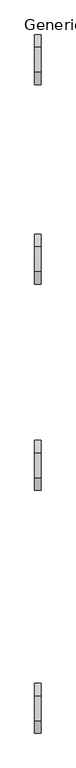
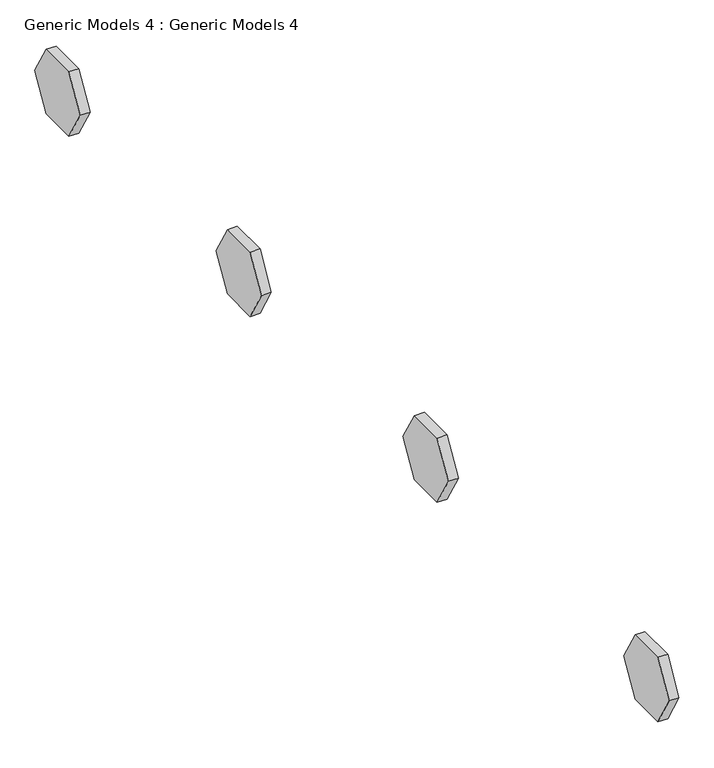
"""IFC4 building model written with IfcOpenShell, lengths in millimetres: proxy geometry, Generic Models 4 : Generic Models 4."""

from ifc_helpers import new_model, si_unit, frame, origin, place, context, project, spatial, polyline, outline, extrude, source, transform, mapped, element, save


def generic_models_4_generic_models_4_89f42e2c(model_context):
    return source(origin(), model_context, "Body", "SweptSolid", [
        extrude(outline(polyline([(9295.4564589, 1201.8685298), (9905.0564589, 1201.8685298), (10209.8564589, 673.9394437), (9905.0564589, 146.0103575), (9295.4564589, 146.0103575), (8990.6564589, 673.9394437), (9295.4564589, 1201.8685298)])), frame((-7992.5513603, 0.0, 0.0), z_axis=(1.0, 0.0, 0.0), x_axis=(0.0, 1.0, 0.0)), (0.0, 0.0, 1.0), 152.4),
        extrude(outline(polyline([(4418.6564589, 1201.8685298), (5028.2564589, 1201.8685298), (5333.0564589, 673.9394437), (5028.2564589, 146.0103575), (4418.6564589, 146.0103575), (4113.8564589, 673.9394437), (4418.6564589, 1201.8685298)])), frame((-7992.5513603, 0.0, 0.0), z_axis=(1.0, 0.0, 0.0), x_axis=(0.0, 1.0, 0.0)), (0.0, 0.0, 1.0), 152.4),
        extrude(outline(polyline([(-610.5435411, 1201.8685298), (-0.9435411, 1201.8685298), (303.8564589, 673.9394437), (-0.9435411, 146.0103575), (-610.5435411, 146.0103575), (-915.3435411, 673.9394437), (-610.5435411, 1201.8685298)])), frame((-7992.5513603, 0.0, 0.0), z_axis=(1.0, 0.0, 0.0), x_axis=(0.0, 1.0, 0.0)), (0.0, 0.0, 1.0), 152.4),
        extrude(outline(polyline([(-6548.4064015, 1201.8685298), (-5938.8064015, 1201.8685298), (-5634.0064015, 673.9394437), (-5938.8064015, 146.0103575), (-6548.4064015, 146.0103575), (-6853.2064015, 673.9394437), (-6548.4064015, 1201.8685298)])), frame((-7992.5513603, 0.0, 0.0), z_axis=(1.0, 0.0, 0.0), x_axis=(0.0, 1.0, 0.0)), (0.0, 0.0, 1.0), 152.4),
    ])


if __name__ == "__main__":
    model = new_model("IFC4")
    model_context = context("Model", 3, world=origin())
    ifc_project = project(units=[si_unit("LENGTHUNIT", "METRE", prefix="MILLI")], contexts=[model_context])
    site = spatial("IfcSite", under=ifc_project)
    building = spatial("IfcBuilding", under=site)
    placement = place(None, origin())
    generic_models_4_generic_models_4_shape = generic_models_4_generic_models_4_89f42e2c(model_context)
    element("IfcBuildingElementProxy", 1, Name="Generic Models 4 : Generic Models 4", ObjectType="Generic Models 4 : Generic Models 4", at=placement, inside=building, context=model_context, shape_type="MappedRepresentation", body=[
        mapped(generic_models_4_generic_models_4_shape, transform((0.0, 0.0, 0.0), x_axis=(1.0, 0.0, 0.0), y_axis=(0.0, 1.0, 0.0), z_axis=(0.0, 0.0, 1.0))),
    ])
    save(model, "model.ifc")

# Revit data of these elements
# Element 1 (IfcBuildingElementProxy, "Generic Models 4 : Generic Models 4")
#   Materials on its faces: "Door - Frame"
# Materials
#   "Door - Frame": colour RGB 118 70 51, transparency 0, Cost = 0
